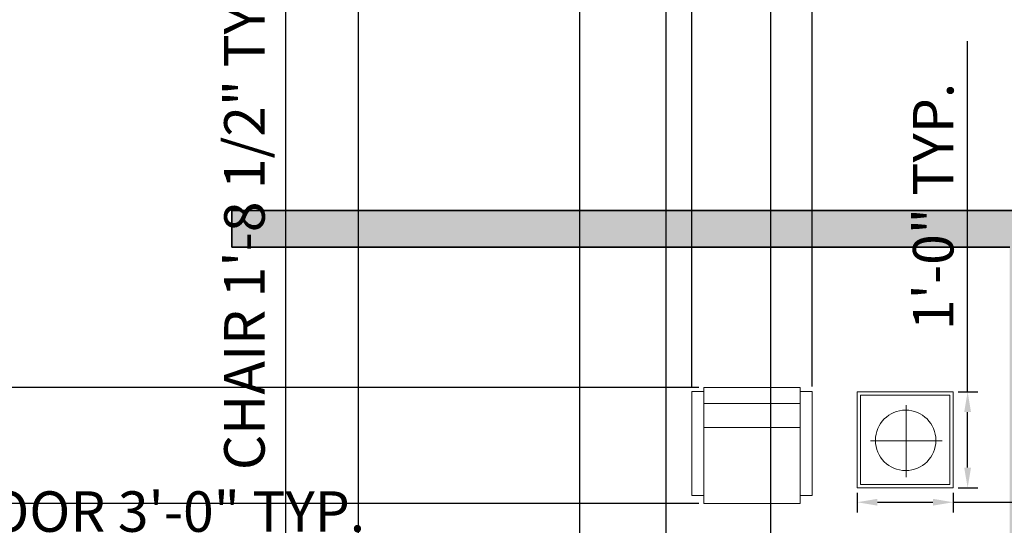
# Model space of a CAD drawing. Units: inches. Extents: x 2923 to 3500, y 1684 to 2381.
# Tile 7 of 12: x 3125 to 3246, y 1930 to 1992. Entities that reach past the tile are written whole.
import ezdxf

# ---------------------------------------------------------------- set-up
doc = ezdxf.new("R2010")
doc.units = ezdxf.units.IN
for name, color, linetype, lineweight in [('A-ANNO-DIMS', 2, 'Continuous', 18), ('A-WALL', 7, 'Continuous', 35), ('A-WALL-PATT', 9, 'Continuous', 13), ('Furniture', 7, 'Continuous', 15)]:
    doc.layers.add(name, color=color, linetype=linetype, lineweight=lineweight)
doc.styles.get("Standard").update_dxf_attribs({"font": 'txt', "height": 5})
doc.dimstyles.new('ISO-25', dxfattribs={"dimtxt": 5, "dimasz": 2.5, "dimexe": 1.25, "dimexo": 0.625, "dimtad": 1, "dimlunit": 3, "dimtxsty": 'Standard', "dimcen": 2.5, "dimadec": 0, "dimazin": 0, "dimtfac": 1, "dimtmove": 0, "dimatfit": 3, "dimfxl": 1, "dimarcsym": 0})

# ---------------------------------------------------------------- blocks, each defined once
blk = doc.blocks.new('TABLE-END')
for p, q in [((0, 0), (0, 11.85)), ((0, 11.85), (11.85, 11.85)), ((0.43, 0.43), (0.43, 11.42)), ((0.43, 11.42), (11.42, 11.42)), ((11.42, 11.42), (11.42, 0.43)), ((11.85, 11.85), (11.85, 0)), ((6.03, 10.2), (6.03, 1.33)), ((10.47, 5.81), (1.63, 5.81)), ((11.85, 0), (0, 0)), ((11.42, 0.43), (0.43, 0.43))]:
    blk.add_line(p, q)
blk.add_circle((5.98, 5.86), 3.73)
blk = doc.blocks.new('*D25')
at = {"layer": 'A-ANNO-DIMS', "color": 0, "lineweight": -2, "transparency": 16777216}
for p, q in [((3069.73, 1931.78), (3069.73, 1925.76)), ((3105.73, 1931.78), (3105.73, 1925.76)), ((3072.23, 1927.01), (3103.23, 1927.01)), ((3105.73, 1927.01), (3174.96, 1927.01))]:
    blk.add_line(p, q, dxfattribs=at)
at = {"layer": 'A-ANNO-DIMS', "color": 0, "transparency": 16777216}
for points in [[(3072.23, 1927.42), (3072.23, 1926.59), (3069.73, 1927.01)], [(3103.23, 1927.42), (3103.23, 1926.59), (3105.73, 1927.01)]]:
    blk.add_solid(points, dxfattribs=at)
at = {"layer": 'Defpoints', "color": 0, "transparency": 16777216}
for p in [(3069.73, 1932.41), (3105.73, 1932.41), (3105.73, 1927.01)]:
    blk.add_point(p, dxfattribs=at)
at = {"layer": 'A-ANNO-DIMS', "color": 0, "transparency": 16777216, "insert": (3141.59, 1930.61), "char_height": 5, "attachment_point": 5}
blk.add_mtext('DOOR 3\'-0" TYP.', dxfattribs=at)
blk = doc.blocks.new('*D39')
at = {"layer": 'A-ANNO-DIMS', "color": 0, "lineweight": -2, "transparency": 16777216}
for p, q in [((3159.85, 2034.29), (3156.13, 2034.29)), ((3157.38, 2031.79), (3157.38, 2016.18)), ((3159.85, 2013.68), (3156.13, 2013.68)), ((3157.38, 2013.68), (3157.38, 1925.17))]:
    blk.add_line(p, q, dxfattribs=at)
at = {"layer": 'A-ANNO-DIMS', "color": 0, "transparency": 16777216}
for points in [[(3156.96, 2031.79), (3157.8, 2031.79), (3157.38, 2034.29)], [(3156.96, 2016.18), (3157.8, 2016.18), (3157.38, 2013.68)]]:
    blk.add_solid(points, dxfattribs=at)
at = {"layer": 'Defpoints', "color": 0, "transparency": 16777216}
for p in [(3160.47, 2034.29), (3157.38, 2013.68), (3160.47, 2013.68)]:
    blk.add_point(p, dxfattribs=at)
at = {"layer": 'A-ANNO-DIMS', "color": 0, "transparency": 16777216, "insert": (3152.94, 1968.18), "char_height": 5, "attachment_point": 5, "rotation": 90}
blk.add_mtext('CHAIR 1\'-8 1/2" TYP.', dxfattribs=at)
blk = doc.blocks.new('*D45')
at = {"layer": 'A-ANNO-DIMS', "color": 0, "lineweight": -2, "transparency": 16777216}
for p, q in [((3227.9, 1933.56), (3227.9, 1931.16)), ((3239.75, 1933.56), (3239.75, 1931.16)), ((3230.4, 1932.41), (3237.25, 1932.41)), ((3239.75, 1932.41), (3310.64, 1932.41))]:
    blk.add_line(p, q, dxfattribs=at)
at = {"layer": 'A-ANNO-DIMS', "color": 0, "transparency": 16777216}
for points in [[(3230.4, 1932.83), (3230.4, 1931.99), (3227.9, 1932.41)], [(3237.25, 1932.83), (3237.25, 1931.99), (3239.75, 1932.41)]]:
    blk.add_solid(points, dxfattribs=at)
at = {"layer": 'Defpoints', "color": 0, "transparency": 16777216}
for p in [(3227.9, 1934.19), (3239.75, 1934.19), (3239.75, 1932.41)]:
    blk.add_point(p, dxfattribs=at)
at = {"layer": 'A-ANNO-DIMS', "color": 0, "transparency": 16777216, "insert": (3276.45, 1936.01), "char_height": 5, "attachment_point": 5}
blk.add_mtext('TABLE 1\'-0" TYP.', dxfattribs=at)
blk = doc.blocks.new('*D46')
at = {"layer": 'A-ANNO-DIMS', "color": 0, "lineweight": -2, "transparency": 16777216}
for p, q in [((3241.53, 1946.04), (3241.53, 1989.31)), ((3240.38, 1946.04), (3242.78, 1946.04)), ((3241.53, 1936.69), (3241.53, 1943.54)), ((3240.38, 1934.19), (3242.78, 1934.19))]:
    blk.add_line(p, q, dxfattribs=at)
at = {"layer": 'A-ANNO-DIMS', "color": 0, "transparency": 16777216}
for points in [[(3241.11, 1943.54), (3241.95, 1943.54), (3241.53, 1946.04)], [(3241.11, 1936.69), (3241.95, 1936.69), (3241.53, 1934.19)]]:
    blk.add_solid(points, dxfattribs=at)
at = {"layer": 'Defpoints', "color": 0, "transparency": 16777216}
for p in [(3239.75, 1946.04), (3241.53, 1946.04), (3239.75, 1934.19)]:
    blk.add_point(p, dxfattribs=at)
at = {"layer": 'A-ANNO-DIMS', "color": 0, "transparency": 16777216, "insert": (3237.93, 1968.92), "char_height": 5, "attachment_point": 5, "rotation": 90}
blk.add_mtext('1\'-0" TYP.', dxfattribs=at)
blk = doc.blocks.new('*D54')
at = {"layer": 'A-ANNO-DIMS', "color": 0, "lineweight": -2, "transparency": 16777216}
for p, q in [((3166.32, 2236.75), (3166.32, 1685.66)), ((3193.64, 2236.75), (3193.64, 1685.66)), ((3168.82, 1686.91), (3191.14, 1686.91)), ((3193.64, 1686.91), (3235.49, 1686.91))]:
    blk.add_line(p, q, dxfattribs=at)
at = {"layer": 'A-ANNO-DIMS', "color": 0, "transparency": 16777216}
for points in [[(3168.82, 1687.32), (3168.82, 1686.49), (3166.32, 1686.91)], [(3191.14, 1687.32), (3191.14, 1686.49), (3193.64, 1686.91)]]:
    blk.add_solid(points, dxfattribs=at)
at = {"layer": 'Defpoints', "color": 0, "transparency": 16777216}
for p in [(3166.32, 2237.38), (3193.64, 2237.38), (3193.64, 1686.91)]:
    blk.add_point(p, dxfattribs=at)
at = {"layer": 'A-ANNO-DIMS', "color": 0, "transparency": 16777216, "insert": (3215.82, 1691.34), "char_height": 5, "attachment_point": 5}
blk.add_mtext('2\'-3 1/2"', dxfattribs=at)
blk = doc.blocks.new('*D62')
at = {"layer": 'A-ANNO-DIMS', "color": 0, "lineweight": -2, "transparency": 16777216}
for p, q in [((3204.33, 1920.39), (3204.33, 2370.16)), ((3217.26, 1920.39), (3217.26, 2370.16)), ((3206.83, 2368.91), (3214.76, 2368.91)), ((3217.26, 2368.91), (3238.87, 2368.91))]:
    blk.add_line(p, q, dxfattribs=at)
at = {"layer": 'A-ANNO-DIMS', "color": 0, "transparency": 16777216}
for points in [[(3206.83, 2369.32), (3206.83, 2368.49), (3204.33, 2368.91)], [(3214.76, 2369.32), (3214.76, 2368.49), (3217.26, 2368.91)]]:
    blk.add_solid(points, dxfattribs=at)
at = {"layer": 'Defpoints', "color": 0, "transparency": 16777216}
for p in [(3217.26, 2368.91), (3204.33, 1919.77), (3217.26, 1919.77)]:
    blk.add_point(p, dxfattribs=at)
at = {"layer": 'A-ANNO-DIMS', "color": 0, "transparency": 16777216, "insert": (3229.31, 2372.51), "char_height": 5, "attachment_point": 5}
blk.add_mtext('1\'-1"', dxfattribs=at)
blk = doc.blocks.new('*D66')
at = {"layer": 'A-ANNO-DIMS', "color": 0, "lineweight": -2, "transparency": 16777216}
for p, q in [((3207.52, 1946.69), (3207.52, 2370.16)), ((3222.33, 1946.69), (3222.33, 2370.16)), ((3210.02, 2368.91), (3219.83, 2368.91)), ((3222.33, 2368.91), (3244.89, 2368.91))]:
    blk.add_line(p, q, dxfattribs=at)
at = {"layer": 'A-ANNO-DIMS', "color": 0, "transparency": 16777216}
for points in [[(3210.02, 2369.32), (3210.02, 2368.49), (3207.52, 2368.91)], [(3219.83, 2369.32), (3219.83, 2368.49), (3222.33, 2368.91)]]:
    blk.add_solid(points, dxfattribs=at)
at = {"layer": 'Defpoints', "color": 0, "transparency": 16777216}
for p in [(3222.33, 2368.91), (3207.52, 1946.07), (3222.33, 1946.07)]:
    blk.add_point(p, dxfattribs=at)
at = {"layer": 'A-ANNO-DIMS', "color": 0, "transparency": 16777216, "insert": (3234.86, 2372.51), "char_height": 5, "attachment_point": 5}
blk.add_mtext('1\'-3"', dxfattribs=at)
blk = doc.blocks.new('*D67')
at = {"layer": 'A-ANNO-DIMS', "color": 0, "lineweight": -2, "transparency": 16777216}
for p, q in [((2934.73, 1946.56), (2934.73, 1987.45)), ((3208.37, 1946.56), (2933.48, 1946.56)), ((2934.73, 1934.74), (2934.73, 1944.06)), ((3208.37, 1932.24), (2933.48, 1932.24))]:
    blk.add_line(p, q, dxfattribs=at)
at = {"layer": 'A-ANNO-DIMS', "color": 0, "transparency": 16777216}
for points in [[(2934.31, 1944.06), (2935.15, 1944.06), (2934.73, 1946.56)], [(2934.31, 1934.74), (2935.15, 1934.74), (2934.73, 1932.24)]]:
    blk.add_solid(points, dxfattribs=at)
at = {"layer": 'Defpoints', "color": 0, "transparency": 16777216}
for p in [(2934.73, 1946.56), (3209, 1946.56), (3209, 1932.24)]:
    blk.add_point(p, dxfattribs=at)
at = {"layer": 'A-ANNO-DIMS', "color": 0, "transparency": 16777216, "insert": (2930.3, 1968.26), "char_height": 5, "attachment_point": 5, "rotation": 90}
blk.add_mtext('1\'-2 1/2"', dxfattribs=at)

msp = doc.modelspace()

# ---------------------------------------------------------------- hatches: boundary and pattern name
at = {"layer": 'A-WALL-PATT'}
h = msp.add_hatch(color=256, dxfattribs=at)
h.dxf.hatch_style = 1
h.paths.add_polyline_path([(3014.23, 2262.406), (2969.23, 2262.406), (2969.23, 2201.5), (2978.23, 2201.5), (2978.23, 2213.699), (2978.23, 2253.406), (3014.23, 2253.406)])
h.paths.add_polyline_path([(3119.23, 2262.406), (3074.23, 2262.406), (3074.23, 2253.406), (3110.23, 2253.406), (3110.23, 2109.406), (3105.73, 2109.406), (3105.73, 2104.906), (3114.73, 2104.906), (3114.73, 2152.906), (3119.23, 2152.906), (3119.23, 2157.406), (3114.73, 2157.406), (3114.73, 2253.406), (3119.23, 2253.406)])
h.paths.add_polyline_path([(3179.98, 2262.406), (3149.23, 2262.406), (3149.23, 2253.406), (3179.98, 2253.406)], flags=0)
h.paths.add_polyline_path([(3295.73, 2262.406), (3215.98, 2262.406), (3215.98, 2253.406), (3246.73, 2253.406), (3246.73, 2157.406), (3149.23, 2157.406), (3149.23, 2152.906), (3246.73, 2152.906), (3246.73, 2149.906), (3251.23, 2149.906), (3251.23, 2253.406), (3295.73, 2253.406)])
h.paths.add_polyline_path([(3397.23, 2262.406), (3343.73, 2262.406), (3343.73, 2253.406), (3349.929, 2253.406), (3388.23, 2253.406), (3388.23, 2199.406), (3397.23, 2199.406)])
h.paths.add_polyline_path([(3369.935, 2334.406), (3264.935, 2334.406), (3264.935, 2262.406), (3269.435, 2262.406), (3269.435, 2329.906), (3365.435, 2329.906), (3365.435, 2262.406), (3369.935, 2262.406)])
h.paths.add_polyline_path([(3096.73, 2334.406), (2991.73, 2334.406), (2991.73, 2262.406), (2996.23, 2262.406), (2996.23, 2329.906), (3092.23, 2329.906), (3092.23, 2262.406), (3096.73, 2262.406)])
h.paths.add_polyline_path([(3397.23, 2163.406), (3388.23, 2163.406), (3388.23, 2109.406), (3251.23, 2109.406), (3251.23, 2113.906), (3246.73, 2113.906), (3246.73, 2092.906), (3251.23, 2092.906), (3251.23, 2104.906), (3435.23, 2104.906), (3435.23, 2080.906), (3444.23, 2080.906), (3444.23, 2109.406), (3397.23, 2109.406)])
h.paths.add_polyline_path([(3444.23, 2044.906), (3435.23, 2044.906), (3435.23, 2020.906), (3251.23, 2020.906), (3251.23, 2032.906), (3246.73, 2032.906), (3246.73, 2016.406), (3251.23, 2016.406), (3287.73, 2016.406), (3287.73, 1968.406), (3287.23, 1968.406), (3287.23, 1963.906), (3296.73, 1963.906), (3296.73, 1968.406), (3292.23, 1968.406), (3292.23, 2016.406), (3388.23, 2016.406), (3388.23, 2004.398), (3397.23, 2004.398), (3397.23, 2016.406), (3444.23, 2016.406)])
h.paths.add_polyline_path([(3397.23, 1980.398), (3388.23, 1980.398), (3388.23, 1979.998), (3388.23, 1969.828), (3388.23, 1968.406), (3326.73, 1968.406), (3326.73, 1963.906), (3388.23, 1963.906), (3388.23, 1913.156), (3397.23, 1913.156)])
h.paths.add_polyline_path([(3251.23, 1968.406), (3150.73, 1968.406), (3150.73, 1963.906), (3246.73, 1963.906), (3246.73, 1826.406), (3230.98, 1826.406), (3230.98, 1817.406), (3251.23, 1817.406), (3251.23, 1963.906)])
h.paths.add_polyline_path([(3114.73, 1968.406), (3105.73, 1968.406), (3105.73, 1963.906), (3110.23, 1963.906), (3110.23, 1817.406), (3119.23, 1817.406), (3119.23, 1826.406), (3114.73, 1826.406)])
h.paths.add_polyline_path([(3069.73, 1968.406), (3066.73, 1968.406), (3066.73, 1972.906), (3062.23, 1972.906), (3062.23, 1968.406), (2978.23, 1968.406), (2978.23, 1989.406), (2969.23, 1989.406), (2969.23, 1912.505), (2978.23, 1912.505), (2978.23, 1925.355), (2978.23, 1963.906), (3069.73, 1963.906)])
h.paths.add_polyline_path([(3066.73, 2104.906), (3069.73, 2104.906), (3069.73, 2109.406), (3057.73, 2109.406), (3057.73, 2104.906), (3062.23, 2104.906), (3062.23, 2038.906), (2978.23, 2038.906), (2978.23, 2059.906), (2969.23, 2059.906), (2969.23, 2013.406), (2978.23, 2013.406), (2978.23, 2034.406), (3062.23, 2034.406), (3062.23, 2002.906), (3066.73, 2002.906)])
h.paths.add_polyline_path([(3027.73, 2109.406), (2978.23, 2109.406), (2978.23, 2165.5), (2969.23, 2165.5), (2969.23, 2083.906), (2978.23, 2083.906), (2978.23, 2104.906), (3027.73, 2104.906)])
h.paths.add_polyline_path([(2978.23, 1876.505), (2969.23, 1876.505), (2969.23, 1817.406), (3014.23, 1817.406), (3014.23, 1826.406), (2978.23, 1826.406)])
h.paths.add_polyline_path([(2996.23, 1817.406), (2991.73, 1817.406), (2991.73, 1745.406), (3096.73, 1745.406), (3096.73, 1817.406), (3092.23, 1817.406), (3092.23, 1749.906), (2996.23, 1749.906)])
h.paths.add_polyline_path([(3289.73, 1826.406), (3251.23, 1826.406), (3251.23, 1817.406), (3289.73, 1817.406)])
h.paths.add_polyline_path([(3397.23, 1877.156), (3388.23, 1877.156), (3388.23, 1864.957), (3388.23, 1826.406), (3349.73, 1826.406), (3349.73, 1817.406), (3397.23, 1817.406)])
h.paths.add_polyline_path([(3374.267, 1817.406), (3369.767, 1817.406), (3369.767, 1749.906), (3273.767, 1749.906), (3273.767, 1817.406), (3269.267, 1817.406), (3269.267, 1745.406), (3374.267, 1745.406)])

# ---------------------------------------------------------------- linework, layer by layer
at = {"layer": 'A-WALL'}
for p, q in [((3150.73, 1963.906), (3150.73, 1968.406)), ((3150.73, 1968.406), (3251.23, 1968.406)), ((3150.73, 1963.906), (3246.73, 1963.906))]:
    msp.add_line(p, q, dxfattribs=at)
at = {"layer": 'Furniture'}
for p, q in [((3220.85, 1946.56), (3209, 1946.56)), ((3209, 1946.56), (3209, 1932.241)), ((3220.85, 1932.241), (3220.85, 1946.56)), ((3209, 1946.066), (3207.519, 1946.066)), ((3207.519, 1946.066), (3207.519, 1933.229)), ((3222.331, 1946.066), (3220.85, 1946.066)), ((3222.331, 1933.229), (3222.331, 1946.066)), ((3220.85, 1944.585), (3209, 1944.585)), ((3209, 1941.622), (3220.85, 1941.622)), ((3207.519, 1933.229), (3209, 1933.229)), ((3220.85, 1933.229), (3222.331, 1933.229)), ((3209, 1932.241), (3220.85, 1932.241))]:
    msp.add_line(p, q, dxfattribs=at)

# ---------------------------------------------------------------- block references
msp.add_blockref('TABLE-END', (3227.902, 1934.187), dxfattribs=at)

# ---------------------------------------------------------------- dimensions: what is measured, and where the dimension line sits
at = {"layer": 'A-ANNO-DIMS'}
for base, p1, p2, picture, middle in [((3217.261, 2368.906), (3204.334, 1919.766), (3217.261, 1919.766), '*D62', (3229.315, 2372.507)), ((3222.331, 2368.906), (3207.519, 1946.066), (3222.331, 1946.066), '*D66', (3234.86, 2372.507)), ((3193.644, 1686.906), (3166.316, 2237.38), (3193.644, 2237.38), '*D54', (3215.817, 1691.341))]:
    dim = msp.add_linear_dim(base=base, p1=p1, p2=p2, dimstyle='ISO-25', override={"dimdec": 1, "dimlfac": 1, "dimrnd": 0, "dimzin": 1, "dimdsep": 46, "dimlunit": 4, "dimfrac": 2}, dxfattribs=at)
    dim.commit()
    dim.dimension.update_dxf_attribs({"geometry": picture, "text_midpoint": middle})
for base, p1, p2, angle, text, picture, middle in [((3157.38, 2013.683), (3160.47, 2034.288), (3160.47, 2013.683), 270, 'CHAIR <> TYP.', '*D39', (3152.945, 1968.177)), ((3241.529, 1946.0372), (3239.7515, 1934.1875), (3239.7515, 1946.0372), 90, '<> TYP.', '*D46', (3237.9278, 1968.9241))]:
    dim = msp.add_linear_dim(base=base, p1=p1, p2=p2, angle=angle, text=text, dimstyle='ISO-25', override={"dimdec": 1, "dimlfac": 1, "dimrnd": 0, "dimzin": 1, "dimdsep": 46, "dimlunit": 4, "dimfrac": 2}, dxfattribs=at)
    dim.commit()
    dim.dimension.update_dxf_attribs({"geometry": picture, "text_midpoint": middle})
dim = msp.add_linear_dim(base=(2934.73, 1946.56), p1=(3209, 1932.241), p2=(3209, 1946.56), angle=90, dimstyle='ISO-25', override={"dimdec": 1, "dimlfac": 1, "dimrnd": 0, "dimzin": 1, "dimdsep": 46, "dimlunit": 4, "dimfrac": 2}, dxfattribs=at)
dim.commit()
dim.dimension.update_dxf_attribs({"geometry": '*D67', "text_midpoint": (2930.295, 1968.256)})
for base, p1, p2, text, picture, middle in [((3239.7515, 1932.41), (3227.9018, 1934.1875), (3239.7515, 1934.1875), 'TABLE <> TYP.', '*D45', (3276.4479, 1936.0112)), ((3105.73, 1927.006), (3069.73, 1932.406), (3105.73, 1932.406), 'DOOR <> TYP.', '*D25', (3141.593, 1930.607))]:
    dim = msp.add_linear_dim(base=base, p1=p1, p2=p2, text=text, dimstyle='ISO-25', override={"dimdec": 1, "dimlfac": 1, "dimrnd": 0, "dimzin": 1, "dimdsep": 46, "dimlunit": 4, "dimfrac": 2}, dxfattribs=at)
    dim.commit()
    dim.dimension.update_dxf_attribs({"geometry": picture, "text_midpoint": middle})

doc.saveas('drawing.dxf')
